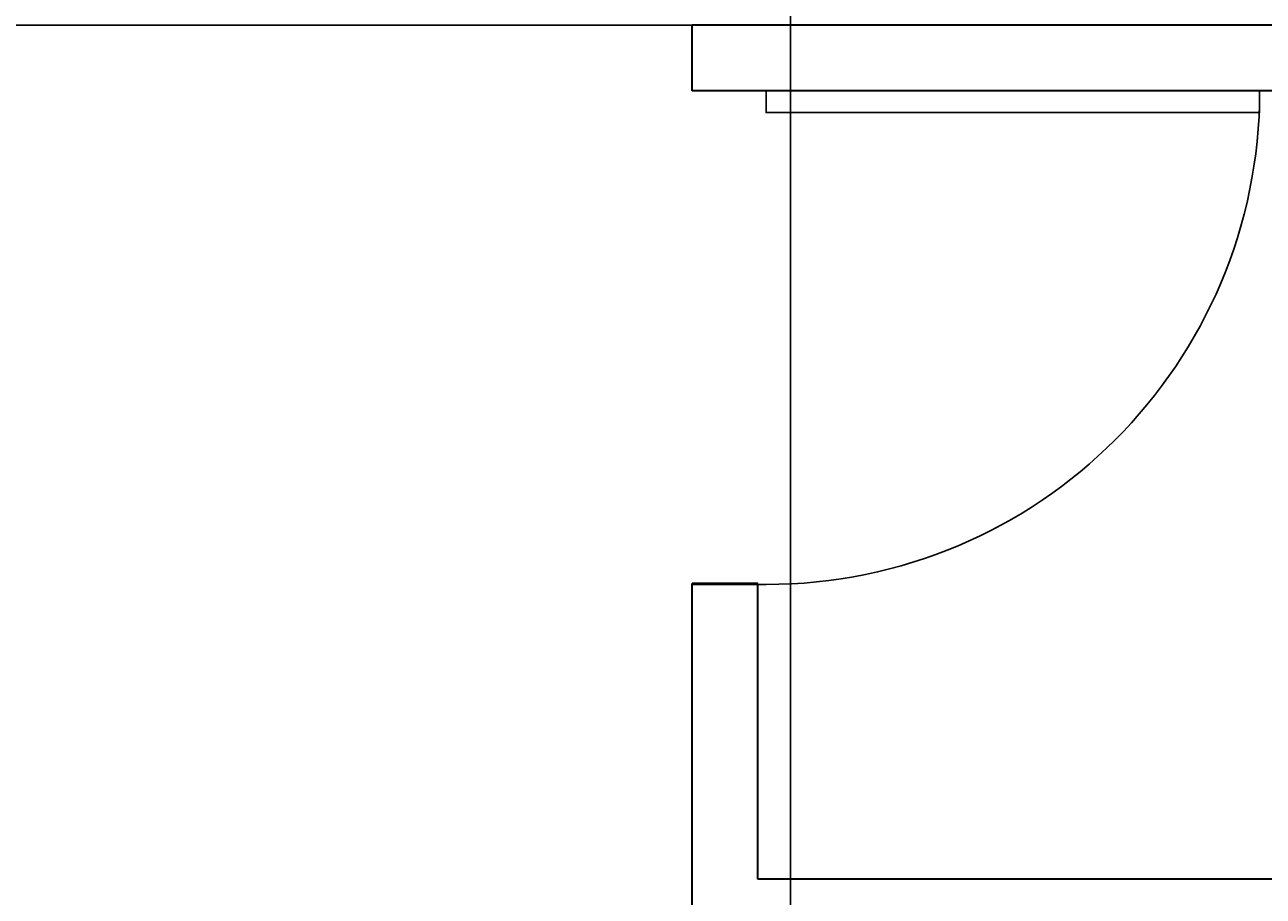
# Model space of a CAD drawing. Units: feet. Extents: x 105 to 1094, y -88 to 588.
# Tile 16 of 59: x 248 to 323, y 301 to 354. Entities that reach past the tile are written whole.
import ezdxf

# ---------------------------------------------------------------- set-up
doc = ezdxf.new("R2010")
doc.units = ezdxf.units.FT
doc.header["$MEASUREMENT"] = 0
for name, color, linetype, lineweight in [('A-ANNO-DIMS', 2, 'Continuous', 18), ('A-DOOR', 3, 'Continuous', 25), ('A-WALL', 7, 'Continuous', 35)]:
    doc.layers.add(name, color=color, linetype=linetype, lineweight=lineweight)
doc.styles.get("Standard").update_dxf_attribs({"font": 'arial.ttf'})
doc.dimstyles.get("Standard").update_dxf_attribs({"dimtxt": 0.18, "dimasz": 0.18, "dimexe": 0.18, "dimexo": 0.0625, "dimgap": 0.09, "dimtad": 0, "dimtih": 1, "dimtoh": 1, "dimdec": 4, "dimzin": 0, "dimdsep": 46, "dimtxsty": 'Standard', "dimcen": 0.09, "dimadec": 0, "dimazin": 0, "dimtfac": 1, "dimtdec": 4, "dimtofl": 0, "dimtmove": 0, "dimatfit": 3, "dimfxl": 1, "dimtolj": 1, "dimtzin": 0, "dimarcsym": 0})

# ---------------------------------------------------------------- blocks, each defined once
blk = doc.blocks.new('*U4')
for p, q in [((0, 0), (0, -6)), ((-40, 0), (-40, -6))]:
    blk.add_line(p, q)
blk.add_lwpolyline([(0, 0), (0, 40), (-1.75, 40), (-1.75, 0)], close=True)
blk.add_arc((0, 0), 40, 90, 180)
blk = doc.blocks.new('*D21')
at = {"layer": 'A-ANNO-DIMS', "color": 0, "lineweight": -2, "transparency": 16777216}
for p, q in [((849.626, 543.081), (105.458, 543.081)), ((105.638, 542.901), (105.638, 250.263)), ((105.638, -42.739), (105.638, 249.899)), ((849.626, -42.919), (105.458, -42.919))]:
    blk.add_line(p, q, dxfattribs=at)
at = {"layer": 'A-ANNO-DIMS', "color": 0, "transparency": 16777216}
for points in [[(105.608, 542.901), (105.668, 542.901), (105.638, 543.081)], [(105.608, -42.739), (105.668, -42.739), (105.638, -42.919)]]:
    blk.add_solid(points, dxfattribs=at)
at = {"layer": 'Defpoints', "color": 0, "transparency": 16777216}
for p in [(105.638, 543.081), (849.688, 543.081), (849.688, -42.919)]:
    blk.add_point(p, dxfattribs=at)
at = {"layer": 'A-ANNO-DIMS', "color": 0, "transparency": 16777216, "insert": (105.638, 250.081), "char_height": 0.18, "attachment_point": 5}
blk.add_mtext('\\A1;586', dxfattribs=at)
blk = doc.blocks.new('*D33')
at = {"layer": 'A-ANNO-DIMS', "color": 0, "lineweight": -2, "transparency": 16777216}
for p, q in [((646.626, 395.081), (105.458, 395.081)), ((105.638, 394.901), (105.638, 345.263)), ((105.638, 295.261), (105.638, 344.899)), ((646.626, 295.081), (105.458, 295.081))]:
    blk.add_line(p, q, dxfattribs=at)
at = {"layer": 'A-ANNO-DIMS', "color": 0, "transparency": 16777216}
for points in [[(105.608, 394.901), (105.668, 394.901), (105.638, 395.081)], [(105.608, 295.261), (105.668, 295.261), (105.638, 295.081)]]:
    blk.add_solid(points, dxfattribs=at)
at = {"layer": 'Defpoints', "color": 0, "transparency": 16777216}
for p in [(646.688, 395.081), (105.638, 295.081), (646.688, 295.081)]:
    blk.add_point(p, dxfattribs=at)
at = {"layer": 'A-ANNO-DIMS', "color": 0, "transparency": 16777216, "insert": (105.638, 345.081), "char_height": 0.18, "attachment_point": 5}
blk.add_mtext('\\A1;100', dxfattribs=at)
blk = doc.blocks.new('*D38')
at = {"layer": 'A-ANNO-DIMS', "color": 0, "lineweight": -2, "transparency": 16777216}
for p, q in [((150.688, 224.144), (150.688, 588.311)), ((294.688, 224.144), (294.688, 588.311)), ((150.868, 588.131), (222.408, 588.131)), ((294.508, 588.131), (222.968, 588.131))]:
    blk.add_line(p, q, dxfattribs=at)
at = {"layer": 'A-ANNO-DIMS', "color": 0, "transparency": 16777216}
for points in [[(150.868, 588.161), (150.868, 588.101), (150.688, 588.131)], [(294.508, 588.161), (294.508, 588.101), (294.688, 588.131)]]:
    blk.add_solid(points, dxfattribs=at)
at = {"layer": 'Defpoints', "color": 0, "transparency": 16777216}
for p in [(294.688, 588.131), (150.688, 224.081), (294.688, 224.081)]:
    blk.add_point(p, dxfattribs=at)
at = {"layer": 'A-ANNO-DIMS', "color": 0, "transparency": 16777216, "insert": (222.688, 588.131), "char_height": 0.18, "attachment_point": 5}
blk.add_mtext('\\A1;144', dxfattribs=at)
blk = doc.blocks.new('*D39')
at = {"layer": 'A-ANNO-DIMS', "color": 0, "lineweight": -2, "transparency": 16777216}
for p, q in [((294.688, 204.144), (294.688, 588.311)), ((370.688, 204.144), (370.688, 588.311)), ((294.868, 588.131), (332.47, 588.131)), ((370.508, 588.131), (332.906, 588.131))]:
    blk.add_line(p, q, dxfattribs=at)
at = {"layer": 'A-ANNO-DIMS', "color": 0, "transparency": 16777216}
for points in [[(294.868, 588.161), (294.868, 588.101), (294.688, 588.131)], [(370.508, 588.161), (370.508, 588.101), (370.688, 588.131)]]:
    blk.add_solid(points, dxfattribs=at)
at = {"layer": 'Defpoints', "color": 0, "transparency": 16777216}
for p in [(370.688, 588.131), (294.688, 204.081), (370.688, 204.081)]:
    blk.add_point(p, dxfattribs=at)
at = {"layer": 'A-ANNO-DIMS', "color": 0, "transparency": 16777216, "insert": (332.688, 588.131), "char_height": 0.18, "attachment_point": 5}
blk.add_mtext('\\A1;76', dxfattribs=at)
blk = doc.blocks.new('*D51')
at = {"layer": 'A-ANNO-DIMS', "color": 0, "lineweight": -2, "transparency": 16777216}
for p, q in [((432.626, 394.081), (105.458, 394.081)), ((105.638, 393.901), (105.638, 374.263)), ((105.638, 354.261), (105.638, 373.899)), ((426.626, 354.081), (105.458, 354.081))]:
    blk.add_line(p, q, dxfattribs=at)
at = {"layer": 'A-ANNO-DIMS', "color": 0, "transparency": 16777216}
for points in [[(105.608, 393.901), (105.668, 393.901), (105.638, 394.081)], [(105.608, 354.261), (105.668, 354.261), (105.638, 354.081)]]:
    blk.add_solid(points, dxfattribs=at)
at = {"layer": 'Defpoints', "color": 0, "transparency": 16777216}
for p in [(432.688, 394.081), (105.638, 354.081), (426.688, 354.081)]:
    blk.add_point(p, dxfattribs=at)
at = {"layer": 'A-ANNO-DIMS', "color": 0, "transparency": 16777216, "insert": (105.638, 374.081), "char_height": 0.18, "attachment_point": 5}
blk.add_mtext('\\A1;40', dxfattribs=at)

msp = doc.modelspace()

# ---------------------------------------------------------------- linework, layer by layer
at = {"layer": 'A-WALL'}
for p, q in [((374.6883, 354.0812), (288.6883, 354.0812)), ((288.6883, 350.0812), (288.6883, 354.0812)), ((370.6883, 350.0812), (288.6883, 350.0812)), ((292.6883, 320.0812), (288.6883, 320.0812)), ((288.6883, 282.0812), (288.6883, 320.0812)), ((292.6883, 302.0812), (292.6883, 320.0812)), ((370.6883, 302.0812), (292.6883, 302.0812))]:
    msp.add_line(p, q, dxfattribs=at)

# ---------------------------------------------------------------- block references
at = {"layer": 'A-DOOR', "xscale": -0.7513941790917756, "yscale": 0.7513941790917756, "zscale": 0.7513941790917756, "rotation": 270}
msp.add_blockref('*U4', (293.1967, 350.0812), dxfattribs=at)

# ---------------------------------------------------------------- dimensions: what is measured, and where the dimension line sits
at = {"layer": 'A-ANNO-DIMS'}
for base, p1, p2, picture, middle in [((294.6883, 588.1312), (150.6883, 224.0812), (294.6883, 224.0812), '*D38', (222.6883, 588.1312)), ((370.6883, 588.1312), (294.6883, 204.0812), (370.6883, 204.0812), '*D39', (332.6883, 588.1312))]:
    dim = msp.add_linear_dim(base=base, p1=p1, p2=p2, dimstyle='Standard', override={"dimdec": 0, "dimlfac": 1, "dimrnd": 0, "dimzin": 0, "dimdsep": 46, "dimlunit": 2}, dxfattribs=at)
    dim.commit()
    dim.dimension.update_dxf_attribs({"geometry": picture, "text_midpoint": middle})
for base, p1, p2, picture, middle in [((105.6383, 543.0812), (849.6883, -42.9188), (849.6883, 543.0812), '*D21', (105.6383, 250.0812)), ((105.6383, 295.0812), (646.6883, 395.0812), (646.6883, 295.0812), '*D33', (105.6383, 345.0812)), ((105.6383, 354.0812), (432.6883, 394.0812), (426.6883, 354.0812), '*D51', (105.6383, 374.0812))]:
    dim = msp.add_linear_dim(base=base, p1=p1, p2=p2, angle=90, dimstyle='Standard', override={"dimdec": 0, "dimlfac": 1, "dimrnd": 0, "dimzin": 0, "dimdsep": 46, "dimlunit": 2}, dxfattribs=at)
    dim.commit()
    dim.dimension.update_dxf_attribs({"geometry": picture, "text_midpoint": middle})

doc.saveas('drawing.dxf')
